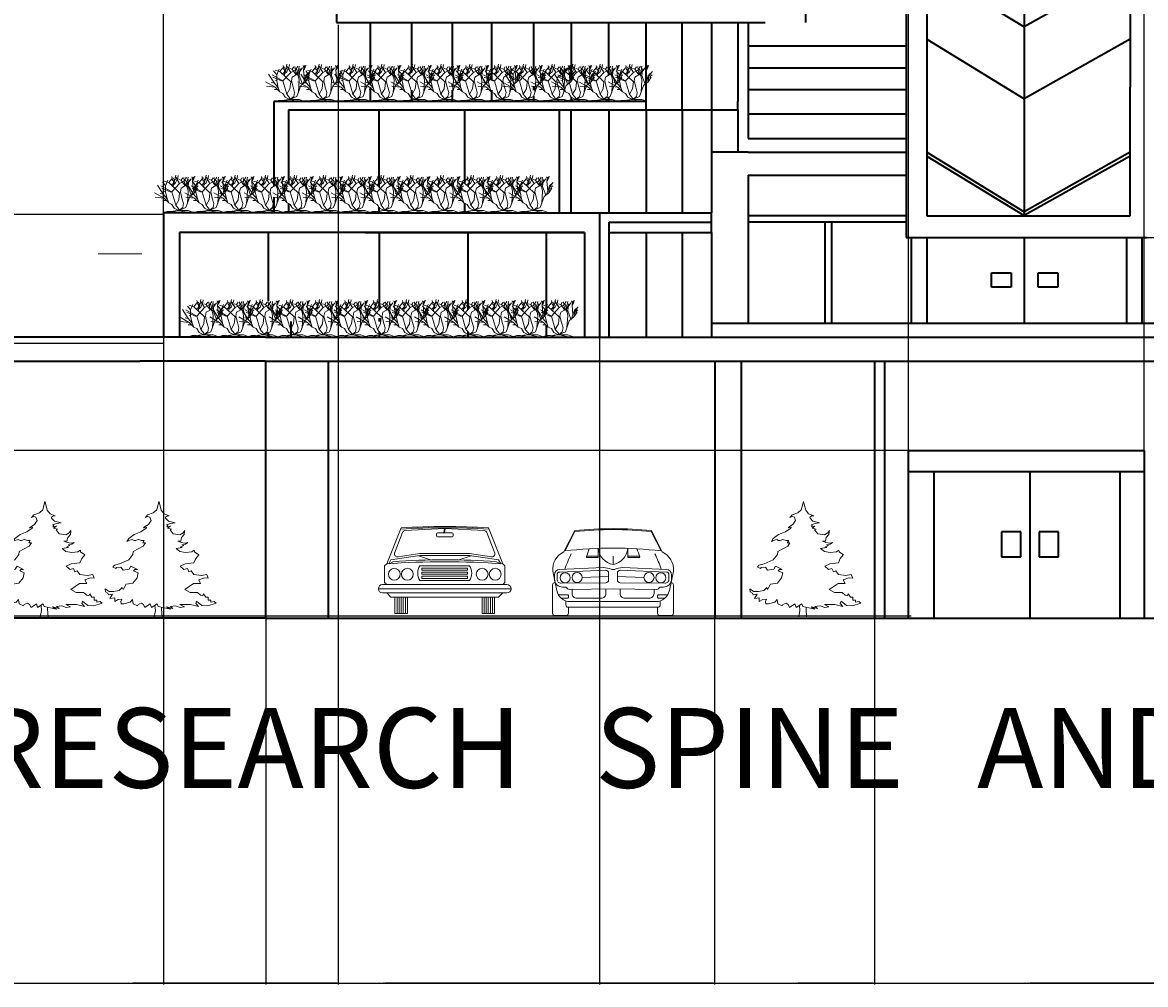
# Model space of a CAD drawing. Units: inches. Extents: x -160 to 434, y -145 to 103.
# Tile 2 of 7: x -26 to 107, y -145 to -31. Entities that reach past the tile are written whole.
import ezdxf

# ---------------------------------------------------------------- set-up
doc = ezdxf.new("R2010")
doc.units = ezdxf.units.IN
doc.header["$MEASUREMENT"] = 0
for name, color, linetype, lineweight in [('A-ANNO-DIMS', 2, 'Continuous', 18), ('A-ANNO-SYMB', 2, 'Continuous', 13), ('A-ANNO-TEXT', 3, 'Continuous', 18), ('A-ELEV', 7, 'Continuous', 35), ('A-ENTO-VEHC', 8, 'Continuous', 13), ('L-PLNT', 3, 'Continuous', 13)]:
    doc.layers.add(name, color=color, linetype=linetype, lineweight=lineweight)
doc.styles.get("Standard").update_dxf_attribs({"font": 'arial.ttf'})
doc.dimstyles.get("Standard").update_dxf_attribs({"dimtxt": 0.18, "dimasz": 0.18, "dimexe": 0.18, "dimexo": 0.0625, "dimgap": 0.09, "dimtad": 0, "dimtih": 1, "dimtoh": 1, "dimdec": 4, "dimzin": 0, "dimdsep": 46, "dimtxsty": 'Standard', "dimcen": 0.09, "dimadec": 0, "dimazin": 0, "dimtfac": 1, "dimtdec": 4, "dimtofl": 0, "dimtmove": 0, "dimatfit": 3, "dimfxl": 1, "dimtolj": 1, "dimtzin": 0, "dimarcsym": 0})

# ---------------------------------------------------------------- blocks, each defined once
blk = doc.blocks.new('*U7')
for p, q in [((-8.263, 7.598), (-8.747, 14.105)), ((-9.75, 0), (-8.263, 7.598)), ((-0.771, 9.56), (-0.69, 11.833)), ((0, 0), (-0.771, 9.56))]:
    blk.add_line(p, q)
for points in [[(-3.9, 142.35), (-6.596, 132.037), (-10.801, 128.443), (-17.81, 126.047), (-20.614, 122.452), (-17.81, 123.65), (-15.007, 123.051), (-13.605, 118.858), (-16.876, 114.065), (-21.549, 111.07), (-22.951, 109.872), (-19.212, 110.471), (-19.68, 109.273), (-26.222, 105.079), (-34.633, 101.485), (-41.175, 96.693), (-43.511, 93.098), (-41.175, 94.296), (-36.969, 95.494), (-34.633, 94.296), (-32.764, 94.296), (-29.493, 95.494)], [(-3.759, 141.97), (-1.074, 131.643), (2.437, 127.141), (8.84, 124.493), (6.568, 124.493), (4.09, 123.169), (4.296, 121.846), (7.807, 117.874), (16.069, 116.02), (10.492, 115.226), (5.535, 113.372), (6.981, 112.843), (5.948, 110.989), (10.286, 112.048), (6.775, 109.401), (11.732, 108.077), (9.873, 107.282), (13.797, 102.516), (21.852, 101.192), (25.983, 103.84), (28.048, 106.488), (27.842, 105.164), (27.429, 101.457), (24.124, 97.75), (23.091, 93.513), (19.58, 93.513), (23.505, 91.66), (28.255, 90.866), (31.973, 91.925), (29.081, 89.806), (24.537, 88.747), (26.809, 88.218), (22.472, 86.099), (24.95, 85.57), (17.308, 84.246), (21.852, 80.804), (29.081, 79.215), (36.723, 80.009), (39.821, 82.392), (40.028, 80.009), (45.398, 76.567)], [(-29.25, 95.55), (-25.287, 94.296), (-22.016, 94.296), (-23.885, 91.301), (-20.614, 91.301), (-23.418, 87.108), (-35.567, 80.518), (-36.035, 76.924), (-41.175, 70.334), (-52.389, 65.542), (-58.931, 63.744), (-60.8, 61.348), (-57.062, 59.551), (-56.128, 60.749), (-50.987, 61.348), (-48.184, 57.754), (-40.707, 58.952), (-38.371, 62.546), (-30.427, 58.353), (-33.698, 58.353), (-35.1, 56.556), (-29.493, 54.159), (-30.894, 48.169), (-36.035, 41.579), (-44.446, 40.381), (-48.184, 33.791), (-49.118, 36.188), (-52.857, 32.593), (-59.399, 31.395), (-65.473, 31.395), (-70.146, 34.39), (-69.679, 30.796), (-66.875, 28.999), (-65.941, 27.202), (-61.268, 27.801), (-64.539, 22.409), (-58.464, 23.607), (-58.464, 18.815), (-54.258, 21.211), (-49.586, 21.81), (-50.987, 18.815), (-50.52, 15.82), (-47.249, 15.82), (-39.306, 18.216), (-36.502, 21.211), (-35.567, 15.82), (-30.427, 13.423), (-29.493, 15.221), (-25.287, 17.018), (-22.951, 15.221), (-21.081, 11.626), (-14.539, 15.82), (-13.138, 11.626), (-6.128, 15.82), (-4.726, 12.824), (10.226, 9.23), (5.554, 12.225), (13.497, 10.428), (10.226, 12.824), (16.768, 13.423), (22.376, 11.626), (27.516, 12.225), (21.909, 15.221), (34.993, 15.221), (44.806, 12.824), (41.535, 16.419), (42.469, 19.414), (49.011, 14.023), (56.487, 13.423), (66.768, 17.018), (64.431, 18.815), (60.226, 18.216), (60.226, 20.612), (56.955, 20.612), (56.955, 24.206), (54.151, 24.206), (51.348, 28.4), (50.413, 26.004), (47.609, 26.603), (43.871, 30.197), (38.731, 30.197), (34.525, 30.197), (27.983, 33.791), (38.731, 40.98), (47.609, 40.98), (45.273, 45.773), (52.282, 48.169), (56.955, 47.57), (55.086, 52.362), (48.544, 51.164), (39.198, 52.362), (35.927, 56.556), (33.123, 55.357), (31.254, 59.551), (27.049, 58.353), (22.376, 62.546), (28.451, 65.542), (39.198, 66.74), (41.535, 72.131), (45.273, 76.325)]]:
    blk.add_lwpolyline(points)
blk = doc.blocks.new('*U8')
for p, q in [((-37.38, 32.04), (-28.11, 55.23)), ((-0.21, 54.74), (-0.67, 52.07)), ((0.21, 54.74), (-0.23, 52.08)), ((37.38, 32.04), (28.11, 55.23)), ((-34.71, 34.71), (-16.02, 37.38)), ((-16.94, 37.24), (-9.08, 34.62)), ((-16.02, 37.38), (0, 37.38)), ((16.02, 37.38), (0, 37.38)), ((16.93, 37.24), (9.08, 34.62)), ((34.71, 34.71), (16.02, 37.38)), ((-38.72, 30.71), (-37.38, 32.04)), ((-38.72, 20.03), (-38.72, 30.71)), ((-36.05, 32.04), (-34.71, 34.71)), ((-35.8, 32.16), (-33.38, 33.38)), ((-16.02, 30.71), (16.02, 30.71)), ((-14.69, 29.37), (14.69, 29.37)), ((-14.69, 28.04), (-14.69, 29.37)), ((14.69, 29.37), (14.69, 28.04)), ((35.8, 32.16), (33.38, 33.38)), ((34.71, 34.71), (36.05, 32.04)), ((38.72, 30.71), (37.38, 32.04)), ((38.72, 20.03), (38.72, 30.71)), ((14.69, 28.04), (-14.69, 28.04)), ((-14.69, 26.7), (14.69, 26.7)), ((-14.69, 25.37), (-14.69, 26.7)), ((14.69, 25.37), (-14.69, 25.37)), ((-14.69, 24.03), (14.69, 24.03)), ((-14.69, 22.7), (-14.69, 24.03)), ((14.69, 22.7), (-14.69, 22.7)), ((14.69, 26.7), (14.69, 25.37)), ((14.69, 24.03), (14.69, 22.7)), ((-42.72, 16.02), (42.72, 16.02)), ((-40.05, 18.69), (40.05, 18.69)), ((-37.38, 18.69), (-38.72, 20.03)), ((16.02, 21.36), (-16.02, 21.36)), ((37.38, 18.69), (38.72, 20.03)), ((40.05, 13.35), (-40.05, 13.35)), ((-37.38, 13.35), (-34.71, 10.68)), ((-34.71, 10.68), (34.71, 10.68)), ((-32.04, 10.68), (-32.04, 0)), ((-30.71, 10.68), (-30.71, 0)), ((-29.37, 0), (-29.37, 10.68)), ((-28.04, 10.68), (-28.04, 0)), ((-26.7, 0), (-26.7, 10.68)), ((-25.37, 10.68), (-25.37, 0)), ((-24.03, 0), (-24.03, 10.68)), ((24.03, 0), (24.03, 10.68)), ((25.37, 0), (25.37, 10.68)), ((26.7, 10.68), (26.7, 0)), ((28.04, 0), (28.04, 10.68)), ((29.37, 10.68), (29.37, 0)), ((30.71, 0), (30.71, 10.68)), ((32.04, 10.68), (32.04, 0)), ((34.71, 10.68), (37.38, 13.35)), ((-32.04, 0), (-24.03, 0)), ((32.04, 0), (24.03, 0))]:
    blk.add_line(p, q)
for points in [[(-27.12, 52.31), (-32.28, 38.89)], [(0, 54.74), (-25.63, 53.46)], [(-5.34, 50.07), (-5.34, 51.4)], [(-4.67, 52.07), (0, 52.07)], [(4.67, 52.07), (0, 52.07)], [(0.01, 54.74), (25.64, 53.45)], [(5.34, 50.07), (5.34, 51.4)], [(27.13, 52.3), (32.28, 38.88)], [(0, 49.4), (-4.67, 49.4)], [(0, 49.4), (4.67, 49.4)], [(-30.06, 36.56), (-16.02, 38.72), (0, 38.72)], [(30.06, 36.54), (16.02, 38.71), (0, 38.72)]]:
    blk.add_lwpolyline(points)
for centre in [(-32.47, 25.37), (-24.06, 25.37), (24.06, 25.37), (32.47, 25.37)]:
    blk.add_circle(centre, 3.8)
for centre, radius, start, end in [((0, -432), 487.32, 86.65721, 93.3419), ((0, -431.24), 487.32, 86.69396, 93.3033), ((-25.37, 51.59), 1.89, 97.4497, 154.9311), ((-4.67, 51.4), 0.668, 93.60832, 178.1081), ((4.67, 51.4), 0.668, 1.89193, 86.39168), ((25.37, 51.57), 1.89, 25.04208, 82.52346), ((-4.67, 50.07), 0.668, 184.4192, 266.4386), ((4.67, 50.07), 0.668, 273.5614, 355.5808), ((-30.43, 38.42), 1.89, 166.5724, 279.9572), ((30.43, 38.41), 1.89, 260.016, 13.40079), ((0, -490.66), 524.03, 85.90918, 94.09081), ((0.67, -399.87), 434.58, 90.08801, 94.49321), ((-8.68, 26.03), 8.7, 147.5288, 212.4712), ((-0.67, -399.87), 434.58, 85.50679, 89.91199), ((8.68, 26.03), 8.7, 327.5288, 32.47119), ((-40.05, 16.02), 2.67, 90, 270), ((40.05, 16.02), 2.67, 270, 90)]:
    blk.add_arc(centre, radius, start, end)
blk = doc.blocks.new('*U9')
for p, q in [((-9.51, 37.84), (-9.51, 43.25)), ((0, 32.82), (0, 38.19)), ((9.51, 37.84), (9.51, 43.25)), ((-19.91, 24.53), (-2.81, 25.14)), ((2.81, 25.14), (19.91, 24.53))]:
    blk.add_line(p, q)
for points in [[(-38.83, 28.63), (-36.22, 16.07, 0.355359), (-27.52, 9), (27.58, 9, 0.355331), (36.28, 16.07), (38.89, 28.63, 0.324597), (31.68, 40.93), (24.69, 54.68, 0.052145), (-24.63, 54.68), (-31.63, 40.93, 0.324597)], [(-24.58, 54.09), (-30.92, 41.61), (-30.92, 41.61, -0.059427), (30.98, 41.61), (24.64, 54.09, 0.05217)], [(-16.8, 37.38), (-9.88, 37.38, 0.414214), (-9.51, 37.75), (-9.51, 37.82, 0.414214), (-9.88, 38.19), (-16.8, 38.19, 0.414214), (-17.17, 37.82), (-17.17, 37.75, 0.414214)], [(16.8, 37.38), (9.88, 37.38, -0.414214), (9.51, 37.75), (9.51, 37.82, -0.414214), (9.88, 38.19), (16.8, 38.19, -0.414214), (17.17, 37.82), (17.17, 37.75, -0.414214)], [(-4.66, 29.17, -0.427329), (-2.81, 27.41), (-2.81, 22.88, -0.410558), (-4.56, 21.11), (-33.36, 20.8, -0.417878), (-36.04, 23.45), (-36.04, 26.26, -0.401219), (-34.35, 28.03)], [(4.66, 29.17, 0.427329), (2.81, 27.41), (2.81, 22.88, 0.410558), (4.56, 21.11), (33.36, 20.8, 0.417878), (36.04, 23.45), (36.04, 26.26, 0.401219), (34.35, 28.03)]]:
    blk.add_lwpolyline(points, format="xyb", close=True)
for points in [[(-6.29, 30.92), (-34.43, 29.71, 0.401219), (-37.73, 26.26), (-37.73, 23.63, 0.414214), (-32.43, 18.34), (-31.07, 18.34, -0.198912), (-29.82, 17.82), (-29.29, 17.29, 0.202778), (-28.01, 16.77), (0, 17.13), (28.01, 16.77, 0.202778), (29.29, 17.29), (29.82, 17.82, -0.198912), (31.07, 18.34), (32.43, 18.34, 0.414214), (37.73, 23.63), (37.73, 26.26, 0.401219), (34.43, 29.71), (6.29, 30.92)], [(6.29, 30.92, 0.105807), (0.87, 29.72, -0.131652), (-0.87, 29.72, 0.105807), (-6.29, 30.92)], [(-28.7, 5.37), (-28.7, 1.48, -0.414214), (-30.18, 0), (-37.41, 0, -0.414214), (-38.89, 1.48), (-38.89, 19.74, -0.414214), (-37.41, 21.22), (-37.29, 21.22)], [(-4.56, 17.07), (-4.56, 14.1, -0.414214), (-7.52, 11.14), (-23.43, 11.14, -0.414214), (-26.39, 14.1), (-26.39, 16.79)], [(4.56, 17.07), (4.56, 14.1, 0.414214), (7.52, 11.14), (23.43, 11.14, 0.414214), (26.39, 14.1), (26.39, 16.79)], [(28.7, 5.37), (28.7, 1.48, 0.414214), (30.18, 0), (37.41, 0, 0.414214), (38.89, 1.48), (38.89, 19.74, 0.414214), (37.41, 21.22), (37.35, 21.22)], [(-35.17, 13.37), (-29.44, 13.37, -0.414214), (-28.7, 12.63), (-28.7, 11.88, -0.414214), (-29.44, 11.14), (-33.31, 11.14)], [(-30.39, 9.47), (-30.39, 6.85, 0.414214), (-28.91, 5.37), (28.91, 5.37, 0.414214), (30.39, 6.85), (30.39, 9.47)], [(35.17, 13.37), (29.44, 13.37, 0.414214), (28.7, 12.63), (28.7, 11.88, 0.414214), (29.44, 11.14), (33.31, 11.14)]]:
    blk.add_lwpolyline(points, format="xyb")
for centre in [(-30.79, 24.36), (-23.15, 24.53), (23.15, 24.53), (30.79, 24.36)]:
    blk.add_circle(centre, 3.24)
for centre, radius, start, end in [((27.74, 11.77), 61.38, 152.82966, 162.90143), ((41.5, 19.77), 61.38, 157.83365, 162.90143), ((2.03, 44.22), 11.58, 184.78179, 259.90449), ((-2.03, 44.22), 11.58, 280.09551, 355.21821), ((-41.5, 19.77), 61.38, 17.09857, 22.16635), ((-27.69, 11.77), 61.38, 17.09857, 27.17034)]:
    blk.add_arc(centre, radius, start, end)
blk = doc.blocks.new('*U5')
for p, q in [((-12.471, 19.775), (-12.898, 22.044)), ((-11.28, 19.619), (-12.104, 21.184)), ((-11.433, 18.289), (-10.457, 22.749)), ((-8.16, 17.76), (-10.56, 21.6)), ((-9.48, 19.775), (-8.992, 22.592)), ((-7.2, 19.68), (-6.24, 21.12)), ((-5.086, 17.741), (-5.513, 21.34)), ((-5.28, 19.2), (-3.84, 21.6)), ((-3.377, 18.602), (-2.888, 21.575)), ((-0.508, 21.888), (-0.081, 20.558)), ((-0.203, 19.149), (0.102, 21.34)), ((-0.02, 20.01), (0.896, 21.105)), ((0.041, 20.714), (1.384, 22.044)), ((0.102, 21.34), (0.835, 21.888)), ((-18.24, 11.04), (-21.755, 16.655)), ((-12.96, 12.48), (-19.68, 16.32)), ((-13.92, 12.48), (-19.2, 14.88)), ((-16.8, 16.32), (-18.72, 18.72)), ((-14.88, 18.24), (-17.76, 19.2)), ((-16.8, 16.32), (-15.36, 19.68)), ((-16.8, 12.48), (-16.8, 16.32)), ((-14.88, 18.24), (-12.96, 20.64)), ((-8.16, 12), (-14.88, 18.24)), ((-13.325, 16.724), (-11.433, 18.289)), ((-12.96, 12.48), (-8.16, 17.76)), ((-11.677, 19.071), (-12.471, 19.775)), ((-12.043, 15.628), (-11.921, 18.836)), ((-11.982, 16.802), (-10.579, 18.054)), ((-11.921, 18.836), (-10.64, 20.401)), ((-10.579, 18.054), (-9.846, 19.697)), ((-7.2, 19.68), (-8.64, 20.16)), ((-8.16, 17.76), (-5.28, 19.2)), ((-7.68, 12.48), (-7.2, 14.88)), ((-4.8, 16.32), (-7.2, 19.68)), ((-7.2, 14.88), (-3.84, 16.8)), ((-3.377, 15.315), (-5.086, 17.819)), ((-2.88, 12.96), (-4.32, 19.68)), ((-3.84, 16.8), (-0.96, 20.64)), ((-2.766, 16.802), (-3.377, 18.602)), ((-2.88, 15.84), (-2.4, 20.16)), ((-0.96, 10.56), (-2.88, 15.84)), ((0.346, 13.203), (-0.203, 19.149)), ((-0.142, 19.384), (0.59, 20.401)), ((0.346, 13.203), (1.323, 16.254)), ((0.96, 12), (1.44, 15.36)), ((0.96, 12), (2.88, 14.88)), ((1.323, 16.254), (3.642, 18.289)), ((1.44, 15.36), (2.88, 17.28)), ((1.92, 13.44), (2.4, 15.36)), ((2.4, 15.36), (3.36, 16.32)), ((-17.76, 8.64), (-23.663, 11.961)), ((-17.76, 8.64), (-23.128, 9.222)), ((-18.24, 11.04), (-20.16, 11.52)), ((-15.84, 8.16), (-18.24, 11.04)), ((-16.32, 7.2), (-18.24, 7.2)), ((-16.8, 12.48), (-17.76, 12.96)), ((-14.88, 5.76), (-17.76, 8.64)), ((-15.84, 8.16), (-16.8, 12.48)), ((-14.88, 5.76), (-15.84, 8.16)), ((-12.96, 12.48), (-13.92, 12.48)), ((-10.56, 4.32), (-12.96, 12.48)), ((-10.56, 4.32), (-8.64, 7.68)), ((-8.64, 7.68), (-8.16, 12)), ((-6.72, 8.64), (-7.68, 12.48)), ((-5.76, 5.28), (-6.72, 8.64)), ((-4.32, 2.88), (-1.92, 9.6)), ((-3.36, 5.28), (-2.88, 12.96)), ((-1.92, 9.6), (0.96, 12)), ((-0.48, 10.8), (0.346, 13.203)), ((-15.84, 0.48), (-17.76, 0)), ((-13.44, 0.48), (-15.84, 0.48)), ((-12.96, 4.8), (-14.88, 5.76)), ((-9.6, 0.96), (-13.44, 0.48)), ((-11.52, 2.4), (-12.96, 4.8)), ((-9.6, 0.96), (-12.96, 0)), ((-8.64, 0.96), (-11.52, 2.4)), ((-8.64, 1.92), (-10.56, 4.32)), ((-9.6, 0.96), (-7.68, 0.96)), ((-8.64, 0.96), (-4.32, 2.88)), ((-8.64, 0.96), (-6.24, 2.88)), ((-8.64, 0.96), (-8.64, 1.92)), ((-8.64, 0.96), (-2.88, 0.96)), ((-7.68, 0.96), (-6.24, 0.48)), ((-6.24, 2.88), (-5.76, 5.28)), ((-6.24, 0.48), (-3.36, 0)), ((-2.88, 0.96), (0, 0))]:
    blk.add_line(p, q)
blk = doc.blocks.new('*D12')
at = {"layer": 'A-ANNO-DIMS', "color": 0, "lineweight": -2, "transparency": 16777216}
for p, q in [((-84.07, -101.41), (-84.07, -144.81)), ((403.75, -101.41), (403.75, -144.81)), ((-83.89, -144.63), (159.44, -144.63)), ((403.57, -144.63), (160.24, -144.63))]:
    blk.add_line(p, q, dxfattribs=at)
at = {"layer": 'A-ANNO-DIMS', "color": 0, "transparency": 16777216}
for points in [[(-83.89, -144.6), (-83.89, -144.66), (-84.07, -144.63)], [(403.57, -144.6), (403.57, -144.66), (403.75, -144.63)]]:
    blk.add_solid(points, dxfattribs=at)
at = {"layer": 'Defpoints', "color": 0, "transparency": 16777216}
for p in [(-84.07, -101.35), (403.75, -101.35), (403.75, -144.63)]:
    blk.add_point(p, dxfattribs=at)
at = {"layer": 'A-ANNO-DIMS', "color": 0, "transparency": 16777216, "insert": (159.84, -144.63), "char_height": 0.18, "attachment_point": 5}
blk.add_mtext('\\A1;487.8', dxfattribs=at)
blk = doc.blocks.new('*D15')
at = {"layer": 'A-ANNO-DIMS', "color": 0, "lineweight": -2, "transparency": 16777216}
for p, q in [((2.83, 44.89), (-114.3, 44.89)), ((-114.12, 44.71), (-114.12, -28.36)), ((-114.12, -101.79), (-114.12, -28.72)), ((-29.6, -101.97), (-114.3, -101.97))]:
    blk.add_line(p, q, dxfattribs=at)
at = {"layer": 'A-ANNO-DIMS', "color": 0, "transparency": 16777216}
for points in [[(-114.15, 44.71), (-114.09, 44.71), (-114.12, 44.89)], [(-114.15, -101.79), (-114.09, -101.79), (-114.12, -101.97)]]:
    blk.add_solid(points, dxfattribs=at)
at = {"layer": 'Defpoints', "color": 0, "transparency": 16777216}
for p in [(-114.12, 44.89), (2.89, 44.89), (-29.54, -101.97)]:
    blk.add_point(p, dxfattribs=at)
at = {"layer": 'A-ANNO-DIMS', "color": 0, "transparency": 16777216, "insert": (-114.12, -28.54), "char_height": 0.18, "attachment_point": 5}
blk.add_mtext('\\A1;146.87', dxfattribs=at)
blk = doc.blocks.new('*D16')
at = {"layer": 'A-ANNO-DIMS', "color": 0, "lineweight": -2, "transparency": 16777216}
for p, q in [((-29.54, -102.04), (-29.54, -144.81)), ((2.66, -101.41), (2.66, -144.81)), ((-29.36, -144.63), (-13.76, -144.63)), ((2.48, -144.63), (-13.12, -144.63))]:
    blk.add_line(p, q, dxfattribs=at)
at = {"layer": 'A-ANNO-DIMS', "color": 0, "transparency": 16777216}
for points in [[(-29.36, -144.6), (-29.36, -144.66), (-29.54, -144.63)], [(2.48, -144.6), (2.48, -144.66), (2.66, -144.63)]]:
    blk.add_solid(points, dxfattribs=at)
at = {"layer": 'Defpoints', "color": 0, "transparency": 16777216}
for p in [(-29.54, -101.97), (2.66, -101.35), (2.66, -144.63)]:
    blk.add_point(p, dxfattribs=at)
at = {"layer": 'A-ANNO-DIMS', "color": 0, "transparency": 16777216, "insert": (-13.44, -144.63), "char_height": 0.18, "attachment_point": 5}
blk.add_mtext('\\A1;32.2', dxfattribs=at)
blk = doc.blocks.new('*D17')
at = {"layer": 'A-ANNO-DIMS', "color": 0, "lineweight": -2, "transparency": 16777216}
for p, q in [((2.66, -101.41), (2.66, -144.81)), ((55.95, -101.41), (55.95, -144.81)), ((2.84, -144.63), (28.91, -144.63)), ((55.77, -144.63), (29.7, -144.63))]:
    blk.add_line(p, q, dxfattribs=at)
at = {"layer": 'A-ANNO-DIMS', "color": 0, "transparency": 16777216}
for points in [[(2.84, -144.6), (2.84, -144.66), (2.66, -144.63)], [(55.77, -144.6), (55.77, -144.66), (55.95, -144.63)]]:
    blk.add_solid(points, dxfattribs=at)
at = {"layer": 'Defpoints', "color": 0, "transparency": 16777216}
for p in [(2.66, -101.35), (55.95, -101.35), (55.95, -144.63)]:
    blk.add_point(p, dxfattribs=at)
at = {"layer": 'A-ANNO-DIMS', "color": 0, "transparency": 16777216, "insert": (29.3, -144.63), "char_height": 0.18, "attachment_point": 5}
blk.add_mtext('\\A1;53.29', dxfattribs=at)
blk = doc.blocks.new('*D18')
at = {"layer": 'A-ANNO-DIMS', "color": 0, "lineweight": -2, "transparency": 16777216}
for p, q in [((55.95, -101.41), (55.95, -144.81)), ((74.92, -101.41), (74.92, -144.81)), ((56.13, -144.63), (65.05, -144.63)), ((74.74, -144.63), (65.82, -144.63))]:
    blk.add_line(p, q, dxfattribs=at)
at = {"layer": 'A-ANNO-DIMS', "color": 0, "transparency": 16777216}
for points in [[(56.13, -144.6), (56.13, -144.66), (55.95, -144.63)], [(74.74, -144.6), (74.74, -144.66), (74.92, -144.63)]]:
    blk.add_solid(points, dxfattribs=at)
at = {"layer": 'Defpoints', "color": 0, "transparency": 16777216}
for p in [(55.95, -101.35), (74.92, -101.35), (74.92, -144.63)]:
    blk.add_point(p, dxfattribs=at)
at = {"layer": 'A-ANNO-DIMS', "color": 0, "transparency": 16777216, "insert": (65.44, -144.63), "char_height": 0.18, "attachment_point": 5}
blk.add_mtext('\\A1;18.97', dxfattribs=at)
blk = doc.blocks.new('*D19')
at = {"layer": 'A-ANNO-DIMS', "color": 0, "lineweight": -2, "transparency": 16777216}
for p, q in [((74.92, -101.41), (74.92, -144.81)), ((111.05, -101.41), (111.05, -144.81)), ((75.1, -144.63), (92.59, -144.63)), ((110.87, -144.63), (93.38, -144.63))]:
    blk.add_line(p, q, dxfattribs=at)
at = {"layer": 'A-ANNO-DIMS', "color": 0, "transparency": 16777216}
for points in [[(75.1, -144.6), (75.1, -144.66), (74.92, -144.63)], [(110.87, -144.6), (110.87, -144.66), (111.05, -144.63)]]:
    blk.add_solid(points, dxfattribs=at)
at = {"layer": 'Defpoints', "color": 0, "transparency": 16777216}
for p in [(74.92, -101.35), (111.05, -101.35), (111.05, -144.63)]:
    blk.add_point(p, dxfattribs=at)
at = {"layer": 'A-ANNO-DIMS', "color": 0, "transparency": 16777216, "insert": (92.98, -144.63), "char_height": 0.18, "attachment_point": 5}
blk.add_mtext('\\A1;36.12', dxfattribs=at)
blk = doc.blocks.new('*D24')
at = {"layer": 'A-ANNO-DIMS', "color": 0, "lineweight": -2, "transparency": 16777216}
for p, q in [((78.96, -81.39), (78.96, 102.5)), ((79.14, 102.32), (92.54, 102.32)), ((106.73, 102.32), (93.33, 102.32)), ((106.91, -81.39), (106.91, 102.5))]:
    blk.add_line(p, q, dxfattribs=at)
at = {"layer": 'A-ANNO-DIMS', "color": 0, "transparency": 16777216}
for points in [[(79.14, 102.35), (79.14, 102.29), (78.96, 102.32)], [(106.73, 102.35), (106.73, 102.29), (106.91, 102.32)]]:
    blk.add_solid(points, dxfattribs=at)
at = {"layer": 'Defpoints', "color": 0, "transparency": 16777216}
for p in [(106.91, 102.32), (78.96, -81.45), (106.91, -81.45)]:
    blk.add_point(p, dxfattribs=at)
at = {"layer": 'A-ANNO-DIMS', "color": 0, "transparency": 16777216, "insert": (92.94, 102.32), "char_height": 0.18, "attachment_point": 5}
blk.add_mtext('\\A1;27.95', dxfattribs=at)
blk = doc.blocks.new('*D25')
at = {"layer": 'A-ANNO-DIMS', "color": 0, "lineweight": -2, "transparency": 16777216}
for p, q in [((78.9, -81.45), (-114.3, -81.45)), ((-114.12, -81.63), (-114.12, -91.1)), ((-114.12, -100.92), (-114.12, -91.46)), ((79.28, -101.1), (-114.3, -101.1))]:
    blk.add_line(p, q, dxfattribs=at)
at = {"layer": 'A-ANNO-DIMS', "color": 0, "transparency": 16777216}
for points in [[(-114.15, -81.63), (-114.09, -81.63), (-114.12, -81.45)], [(-114.15, -100.92), (-114.09, -100.92), (-114.12, -101.1)]]:
    blk.add_solid(points, dxfattribs=at)
at = {"layer": 'Defpoints', "color": 0, "transparency": 16777216}
for p in [(78.96, -81.45), (-114.12, -101.1), (79.34, -101.1)]:
    blk.add_point(p, dxfattribs=at)
at = {"layer": 'A-ANNO-DIMS', "color": 0, "transparency": 16777216, "insert": (-114.12, -91.28), "char_height": 0.18, "attachment_point": 5}
blk.add_mtext('\\A1;19.646', dxfattribs=at)
blk = doc.blocks.new('*D30')
at = {"layer": 'A-ANNO-DIMS', "color": 0, "lineweight": -2, "transparency": 16777216}
for p, q in [((2.83, 3.66), (-114.3, 3.66)), ((-114.12, 3.48), (-114.12, -32.35)), ((-114.12, -68.55), (-114.12, -32.72)), ((-9.37, -68.73), (-114.3, -68.73))]:
    blk.add_line(p, q, dxfattribs=at)
at = {"layer": 'A-ANNO-DIMS', "color": 0, "transparency": 16777216}
for points in [[(-114.15, 3.48), (-114.09, 3.48), (-114.12, 3.66)], [(-114.15, -68.55), (-114.09, -68.55), (-114.12, -68.73)]]:
    blk.add_solid(points, dxfattribs=at)
at = {"layer": 'Defpoints', "color": 0, "transparency": 16777216}
for p in [(-114.12, 3.66), (2.89, 3.66), (-9.31, -68.73)]:
    blk.add_point(p, dxfattribs=at)
at = {"layer": 'A-ANNO-DIMS', "color": 0, "transparency": 16777216, "insert": (-114.12, -32.54), "char_height": 0.18, "attachment_point": 5}
blk.add_mtext('\\A1;72.4', dxfattribs=at)
blk = doc.blocks.new('*D32')
at = {"layer": 'A-ANNO-DIMS', "color": 0, "lineweight": -2, "transparency": 16777216}
for p, q in [((107.33, -56.17), (433.98, -56.17)), ((433.8, -56.35), (433.8, -61.07)), ((433.8, -66.15), (433.8, -61.43)), ((106.73, -66.33), (433.98, -66.33))]:
    blk.add_line(p, q, dxfattribs=at)
at = {"layer": 'A-ANNO-DIMS', "color": 0, "transparency": 16777216}
for points in [[(433.77, -56.35), (433.83, -56.35), (433.8, -56.17)], [(433.77, -66.15), (433.83, -66.15), (433.8, -66.33)]]:
    blk.add_solid(points, dxfattribs=at)
at = {"layer": 'Defpoints', "color": 0, "transparency": 16777216}
for p in [(107.27, -56.17), (106.67, -66.33), (433.8, -66.33)]:
    blk.add_point(p, dxfattribs=at)
at = {"layer": 'A-ANNO-DIMS', "color": 0, "transparency": 16777216, "insert": (433.8, -61.25), "char_height": 0.18, "attachment_point": 5}
blk.add_mtext('\\A1;10.165', dxfattribs=at)
blk = doc.blocks.new('*D35')
at = {"layer": 'A-ANNO-DIMS', "color": 0, "lineweight": -2, "transparency": 16777216}
for p, q in [((42.27, -53.31), (42.27, -144.81)), ((-9.45, -53.49), (-9.45, -144.81)), ((-9.27, -144.63), (16.02, -144.63)), ((42.09, -144.63), (16.8, -144.63))]:
    blk.add_line(p, q, dxfattribs=at)
at = {"layer": 'A-ANNO-DIMS', "color": 0, "transparency": 16777216}
for points in [[(-9.27, -144.6), (-9.27, -144.66), (-9.45, -144.63)], [(42.09, -144.6), (42.09, -144.66), (42.27, -144.63)]]:
    blk.add_solid(points, dxfattribs=at)
at = {"layer": 'Defpoints', "color": 0, "transparency": 16777216}
for p in [(42.27, -53.24), (-9.45, -53.43), (42.27, -144.63)]:
    blk.add_point(p, dxfattribs=at)
at = {"layer": 'A-ANNO-DIMS', "color": 0, "transparency": 16777216, "insert": (16.41, -144.63), "char_height": 0.18, "attachment_point": 5}
blk.add_mtext('\\A1;51.72', dxfattribs=at)
blk = doc.blocks.new('*D36')
at = {"layer": 'A-ANNO-DIMS', "color": 0, "lineweight": -2, "transparency": 16777216}
for p, q in [((-9.51, -53.43), (-114.3, -53.43)), ((-114.12, -53.61), (-114.12, -60.9)), ((-114.12, -68.55), (-114.12, -61.26)), ((-9.37, -68.73), (-114.3, -68.73))]:
    blk.add_line(p, q, dxfattribs=at)
at = {"layer": 'A-ANNO-DIMS', "color": 0, "transparency": 16777216}
for points in [[(-114.15, -53.61), (-114.09, -53.61), (-114.12, -53.43)], [(-114.15, -68.55), (-114.09, -68.55), (-114.12, -68.73)]]:
    blk.add_solid(points, dxfattribs=at)
at = {"layer": 'Defpoints', "color": 0, "transparency": 16777216}
for p in [(-9.45, -53.43), (-114.12, -68.73), (-9.31, -68.73)]:
    blk.add_point(p, dxfattribs=at)
at = {"layer": 'A-ANNO-DIMS', "color": 0, "transparency": 16777216, "insert": (-114.12, -61.08), "char_height": 0.18, "attachment_point": 5}
blk.add_mtext('\\A1;15.304', dxfattribs=at)
blk = doc.blocks.new('*D37')
at = {"layer": 'A-ANNO-DIMS', "color": 0, "lineweight": -2, "transparency": 16777216}
for p, q in [((11.28, -30.92), (11.28, -144.81)), ((-9.45, -53.49), (-9.45, -144.81)), ((-9.27, -144.63), (0.52, -144.63)), ((11.1, -144.63), (1.31, -144.63))]:
    blk.add_line(p, q, dxfattribs=at)
at = {"layer": 'A-ANNO-DIMS', "color": 0, "transparency": 16777216}
for points in [[(-9.27, -144.6), (-9.27, -144.66), (-9.45, -144.63)], [(11.1, -144.6), (11.1, -144.66), (11.28, -144.63)]]:
    blk.add_solid(points, dxfattribs=at)
at = {"layer": 'Defpoints', "color": 0, "transparency": 16777216}
for p in [(11.28, -30.86), (-9.45, -53.43), (11.28, -144.63)]:
    blk.add_point(p, dxfattribs=at)
at = {"layer": 'A-ANNO-DIMS', "color": 0, "transparency": 16777216, "insert": (0.92, -144.63), "char_height": 0.18, "attachment_point": 5}
blk.add_mtext('\\A1;20.73', dxfattribs=at)
blk = doc.blocks.new('*D47')
at = {"layer": 'A-ANNO-DIMS', "color": 0, "lineweight": -2, "transparency": 16777216}
for p, q in [((-30.07, -67.91), (-30.07, 102.5)), ((-29.89, 102.32), (-20.23, 102.32)), ((-9.63, 102.32), (-19.3, 102.32)), ((-9.45, -53.37), (-9.45, 102.5))]:
    blk.add_line(p, q, dxfattribs=at)
at = {"layer": 'A-ANNO-DIMS', "color": 0, "transparency": 16777216}
for points in [[(-29.89, 102.35), (-29.89, 102.29), (-30.07, 102.32)], [(-9.63, 102.35), (-9.63, 102.29), (-9.45, 102.32)]]:
    blk.add_solid(points, dxfattribs=at)
at = {"layer": 'Defpoints', "color": 0, "transparency": 16777216}
for p in [(-9.45, 102.32), (-9.45, -53.43), (-30.07, -67.97)]:
    blk.add_point(p, dxfattribs=at)
at = {"layer": 'A-ANNO-DIMS', "color": 0, "transparency": 16777216, "insert": (-19.76, 102.32), "char_height": 0.18, "attachment_point": 5}
blk.add_mtext('\\A1;20.625', dxfattribs=at)

msp = doc.modelspace()

# ---------------------------------------------------------------- linework, layer by layer
at = {"layer": 'A-ANNO-SYMB'}
msp.add_line((-17.2202, -58.1074), (-12.0372, -58.1074), dxfattribs=at)
at = {"layer": 'A-ELEV'}
for p, q in [((105.2782, 6.4991), (105.2782, -38.311)), ((78.691, -2.0014), (78.691, -56.1669)), ((81.1405, -2.0014), (81.1405, -53.5674)), ((92.6738, -2.0014), (92.6738, -53.5674)), ((11.0861, -9.1182), (11.0861, -30.6379)), ((66.7815, -30.6379), (66.7815, -24.7325)), ((81.1405, -24.1029), (92.6738, -31.1677)), ((105.2782, -24.1029), (92.6738, -31.1677)), ((11.0861, -30.6379), (61.9316, -30.6379)), ((15.067, -30.6379), (15.067, -37.2498)), ((19.9544, -30.6379), (19.9544, -36.5858)), ((24.8102, -30.6379), (24.8102, -36.9732)), ((29.4459, -30.6379), (29.4459, -37.4933)), ((34.4496, -30.6379), (34.4496, -36.7871)), ((38.9382, -30.6379), (38.9382, -37.5554)), ((43.3532, -30.6379), (43.3532, -36.908)), ((47.7681, -30.6379), (47.7681, -38.6671)), ((47.7681, -30.6379), (47.7681, -41.0229)), ((52.036, -30.6379), (52.036, -38.6671)), ((52.036, -30.6379), (52.036, -41.0229)), ((55.5639, -30.6379), (55.5639, -53.2447)), ((58.6862, -30.6379), (58.6862, -38.6671)), ((59.9278, -30.6379), (59.9278, -38.6671)), ((81.1405, -32.6275), (92.6738, -39.6923)), ((105.2782, -32.6275), (92.6738, -39.6923)), ((59.9278, -33.4031), (78.691, -33.4031)), ((19.9544, -37.1469), (19.9544, -37.1737)), ((59.9278, -36.0223), (78.691, -36.0223)), ((15.067, -37.4944), (15.067, -37.9924)), ((15.067, -38.3382), (15.067, -38.6671)), ((24.8102, -37.9411), (24.8102, -38.2411)), ((34.4496, -38.2245), (34.4496, -38.6671)), ((38.9382, -38.6392), (38.9382, -38.6671)), ((59.9278, -38.6), (78.691, -38.6)), ((105.2782, -53.5674), (105.2782, -38.311)), ((15.067, -38.6671), (15.067, -40.0106)), ((19.9544, -38.6671), (19.9544, -40.0106)), ((24.8102, -38.6671), (24.8102, -40.0106)), ((29.4459, -38.6671), (29.4459, -40.0106)), ((34.4496, -39.3781), (34.4496, -40.0106)), ((38.9382, -39.5312), (38.9382, -40.0106)), ((43.3532, -39.508), (43.3532, -40.0106)), ((58.6862, -38.6671), (58.6862, -40.0106)), ((59.9278, -38.6671), (59.9278, -44.3998)), ((3.6399, -40.0106), (3.6399, -41.0229)), ((47.7681, -40.0106), (3.6399, -40.0106)), ((3.6399, -41.0229), (3.6399, -50.073)), ((5.3878, -41.0229), (47.7681, -41.0229)), ((5.3878, -41.0229), (5.3878, -49.8008)), ((16.0957, -41.0229), (16.0957, -50.1598)), ((26.2769, -41.0229), (26.2769, -49.7194)), ((37.5113, -41.0229), (37.5113, -53.2447)), ((38.9382, -53.2447), (38.9382, -41.0229)), ((43.4443, -53.2447), (43.4443, -41.0229)), ((47.7681, -41.0229), (58.6862, -41.0229)), ((47.8728, -53.2447), (47.8728, -41.0229)), ((52.1459, -53.2447), (52.1459, -41.0229)), ((58.6862, -41.0229), (58.6862, -40.0106)), ((58.6862, -41.0229), (58.6862, -46.0109)), ((59.9278, -41.4999), (78.691, -41.4999)), ((59.9278, -44.3998), (78.691, -44.3998)), ((59.9278, -46.0109), (55.5639, -46.0109)), ((59.9278, -46.0109), (78.691, -46.0109)), ((81.1405, -46.03), (92.6738, -53.0948)), ((81.1405, -46.4882), (92.6738, -53.553)), ((105.2782, -46.03), (92.6738, -53.0948)), ((105.2782, -46.4882), (92.6738, -53.553)), ((59.9278, -48.7744), (59.9278, -66.3322)), ((59.9278, -48.7744), (78.691, -48.7744)), ((5.3878, -50.6359), (5.3878, -50.7427)), ((26.2769, -50.5858), (26.2769, -50.7029)), ((3.6399, -51.3759), (3.6399, -53.2447)), ((14.4937, -53.2447), (-9.473, -53.2447)), ((-6.3978, -53.2447), (-9.473, -53.2447)), ((-9.473, -53.2447), (-9.473, -67.9742)), ((3.6399, -52.675), (3.6399, -53.2447)), ((5.3878, -52.1272), (5.3878, -53.2447)), ((14.4937, -53.2447), (42.2691, -53.2447)), ((16.0957, -52.5428), (16.0957, -53.2447)), ((26.2769, -52.0834), (26.2769, -53.2447)), ((42.2691, -53.2447), (42.2691, -67.9742)), ((42.2691, -53.2447), (55.5639, -53.2447)), ((55.5639, -55.5766), (55.5639, -53.2447)), ((43.4443, -54.3521), (55.5639, -54.3521)), ((43.4443, -55.5766), (43.4443, -54.3521)), ((78.691, -53.5674), (59.9278, -53.5674)), ((78.691, -54.3391), (59.9278, -54.3391)), ((69.0088, -54.3391), (69.0088, -66.3322)), ((69.8034, -54.3391), (69.8034, -66.3322)), ((81.1405, -53.5674), (105.2782, -53.5674)), ((-7.5654, -55.5766), (-7.5654, -67.9742)), ((40.5131, -55.5766), (-7.5654, -55.5766)), ((-6.3978, -55.5766), (-6.9454, -55.5766)), ((2.9669, -55.5766), (2.9669, -63.7195)), ((14.4937, -55.5766), (40.5131, -55.5766)), ((16.1323, -55.5766), (16.1323, -64.7192)), ((26.6646, -55.5766), (26.6646, -64.703)), ((35.9681, -55.5766), (35.9681, -64.4967)), ((40.5131, -55.5766), (40.5131, -67.9742)), ((43.4443, -67.9742), (43.4443, -55.5766)), ((43.4443, -55.5766), (55.5639, -55.5766)), ((47.8728, -67.9742), (47.8728, -55.5766)), ((52.1459, -67.9742), (52.1459, -55.5766)), ((55.5639, -55.5766), (55.5639, -67.9742)), ((78.691, -56.1669), (107.2684, -56.1669)), ((79.2907, -56.1669), (79.2907, -66.3322)), ((81.1405, -56.1669), (81.1405, -66.3322)), ((92.6738, -56.1669), (92.6738, -66.3322)), ((104.8174, -56.1669), (104.8174, -66.3322)), ((106.6672, -56.1669), (106.6672, -66.3322)), ((88.7955, -60.3692), (91.1349, -60.3692)), ((88.7955, -62.0486), (88.7955, -60.3692)), ((91.1349, -60.3692), (91.1349, -62.0486)), ((94.3434, -60.3692), (96.6827, -60.3692)), ((94.3434, -62.0486), (94.3434, -60.3692)), ((96.6827, -60.3692), (96.6827, -62.0486)), ((91.1349, -62.0486), (88.7955, -62.0486)), ((96.6827, -62.0486), (94.3434, -62.0486)), ((3.9379, -64.8024), (3.9379, -65.8042)), ((35.9681, -65.0634), (35.9681, -65.084)), ((-7.5654, -65.6451), (-7.5654, -67.9742)), ((5.6473, -66.1157), (5.6473, -67.9845)), ((16.1323, -65.7443), (16.1323, -66.1335)), ((35.9681, -66.5457), (35.9681, -67.9742)), ((55.5639, -66.3322), (131.6105, -66.3322)), ((-12.2824, -67.9742), (-30.0745, -67.9742)), ((2.6577, -67.9742), (-12.2824, -67.9742)), ((2.6577, -67.9742), (206.9244, -67.9742)), ((2.9669, -67.4341), (2.9669, -67.9742)), ((16.1323, -67.342), (16.1323, -67.9742)), ((26.6646, -67.3028), (26.6646, -67.9742)), ((-30.0745, -70.8373), (-12.2824, -70.8373)), ((2.6577, -70.8373), (-12.2824, -70.8373)), ((2.6577, -70.8373), (206.9244, -70.8373)), ((2.6577, -70.8373), (2.6577, -101.346)), ((10.0595, -70.8373), (10.0595, -101.346)), ((55.9512, -70.8373), (55.9512, -101.346)), ((59.0997, -70.8373), (59.0997, -101.346)), ((74.9222, -70.8373), (74.9222, -101.346)), ((76.1164, -70.8373), (76.1164, -101.346)), ((78.9633, -101.346), (78.9633, -81.4546)), ((78.9633, -81.4546), (106.9124, -81.4546)), ((106.9124, -81.4546), (106.9124, -101.346)), ((78.9633, -83.9177), (106.9124, -83.9177)), ((82.0165, -101.346), (82.0165, -83.9177)), ((93.4076, -101.346), (93.4076, -83.9177)), ((104.094, -101.346), (104.094, -83.9177)), ((89.9978, -91.0851), (89.9978, -94.0578)), ((92.3044, -91.0851), (89.9978, -91.0851)), ((92.3044, -94.0578), (92.3044, -91.0851)), ((94.4622, -91.0851), (94.4622, -94.0578)), ((96.7688, -91.0851), (94.4622, -91.0851)), ((96.7688, -94.0578), (96.7688, -91.0851)), ((89.9978, -94.0578), (92.3044, -94.0578)), ((94.4622, -94.0578), (96.7688, -94.0578)), ((2.6577, -101.346), (-84.0722, -101.346)), ((2.6577, -101.346), (403.7477, -101.346))]:
    msp.add_line(p, q, dxfattribs=at)

# ---------------------------------------------------------------- block references
at = {"layer": 'A-ENTO-VEHC', "xscale": 0.1843091790693797, "yscale": 0.1843091790693797, "zscale": 0.1843091790693797}
for name, p in [('*U8', (23.915, -100.7948)), ('*U9', (43.8866, -101.0241))]:
    msp.add_blockref(name, p, dxfattribs=at)
at = {"layer": 'L-PLNT'}
for name, p, xscale, yscale, zscale in [('*U5', (7.2005, -39.9747), 0.1923638725067976, 0.1923638725067976, 0.1923638725067976), ('*U5', (11.0298, -39.9747), 0.1923638725067976, 0.1923638725067976, 0.1923638725067976), ('*U5', (15.0437, -39.9747), 0.1923638725067976, 0.1923638725067976, 0.1923638725067976), ('*U5', (18.4579, -39.9747), 0.1923638725067976, 0.1923638725067976, 0.1923638725067976), ('*U5', (22.0835, -39.9747), 0.1923638725067976, 0.1923638725067976, 0.1923638725067976), ('*U5', (25.4976, -39.9747), 0.1923638725067976, 0.1923638725067976, 0.1923638725067976), ('*U5', (28.8871, -39.9747), 0.1923638725067976, 0.1923638725067976, 0.1923638725067976), ('*U5', (32.3012, -39.9747), 0.1923638725067976, 0.1923638725067976, 0.1923638725067976), ('*U5', (35.2654, -39.9747), 0.1923638725067976, 0.1923638725067976, 0.1923638725067976), ('*U5', (38.6795, -39.9747), 0.1923638725067976, 0.1923638725067976, 0.1923638725067976), ('*U5', (41.1179, -39.9747), 0.1923638725067976, 0.1923638725067976, 0.1923638725067976), ('*U5', (44.3806, -39.9747), 0.1923638725067976, 0.1923638725067976, 0.1923638725067976), ('*U5', (47.8763, -39.9747), 0.1923638725067976, 0.1923638725067976, 0.1923638725067976), ('*U5', (-5.9892, -53.1486), 0.1923638725067976, 0.1923638725067976, 0.1923638725067976), ('*U5', (-2.3813, -53.1486), 0.1923638725067976, 0.1923638725067976, 0.1923638725067976), ('*U5', (1.0439, -53.1486), 0.1923638725067976, 0.1923638725067976, 0.1923638725067976), ('*U5', (4.6517, -53.1486), 0.1923638725067976, 0.1923638725067976, 0.1923638725067976), ('*U5', (8.0769, -53.1486), 0.1923638725067976, 0.1923638725067976, 0.1923638725067976), ('*U5', (11.5478, -53.1486), 0.1923638725067976, 0.1923638725067976, 0.1923638725067976), ('*U5', (14.9729, -53.1486), 0.1923638725067976, 0.1923638725067976, 0.1923638725067976), ('*U5', (18.3981, -53.1486), 0.1923638725067976, 0.1923638725067976, 0.1923638725067976), ('*U5', (21.9147, -53.1486), 0.1923638725067976, 0.1923638725067976, 0.1923638725067976), ('*U5', (25.4769, -53.1486), 0.1923638725067976, 0.1923638725067976, 0.1923638725067976), ('*U5', (29.0536, -53.1486), 0.1923638725067976, 0.1923638725067976, 0.1923638725067976), ('*U5', (32.5245, -53.1486), 0.1923638725067976, 0.1923638725067976, 0.1923638725067976), ('*U5', (36.0867, -53.1486), 0.1923638725067976, 0.1923638725067976, 0.1923638725067976), ('*U5', (-3.0108, -67.8884), 0.1923638725067976, 0.1923638725067976, 0.1923638725067976), ('*U5', (0.5971, -67.8884), 0.1923638725067976, 0.1923638725067976, 0.1923638725067976), ('*U5', (4.0223, -67.8884), 0.1923638725067976, 0.1923638725067976, 0.1923638725067976), ('*U5', (7.6301, -67.8884), 0.1923638725067976, 0.1923638725067976, 0.1923638725067976), ('*U5', (11.0553, -67.8884), 0.1923638725067976, 0.1923638725067976, 0.1923638725067976), ('*U5', (14.5262, -67.8884), 0.1923638725067976, 0.1923638725067976, 0.1923638725067976), ('*U5', (17.9514, -67.8884), 0.1923638725067976, 0.1923638725067976, 0.1923638725067976), ('*U5', (21.3766, -67.8884), 0.1923638725067976, 0.1923638725067976, 0.1923638725067976), ('*U5', (24.8931, -67.8884), 0.1923638725067976, 0.1923638725067976, 0.1923638725067976), ('*U5', (28.4553, -67.8884), 0.1923638725067976, 0.1923638725067976, 0.1923638725067976), ('*U5', (32.032, -67.8884), 0.1923638725067976, 0.1923638725067976, 0.1923638725067976), ('*U5', (35.5029, -67.8884), 0.1923638725067976, 0.1923638725067976, 0.1923638725067976), ('*U5', (39.0651, -67.8884), 0.1923638725067976, 0.1923638725067976, 0.1923638725067976), ('*U7', (-23.1588, -101.1712), 0.0961203238098615, 0.0961203238098615, 0.0961203238098615), ('*U7', (-9.6368, -101.1712), 0.0961203238098615, 0.0961203238098615, 0.0961203238098615), ('*U7', (66.8677, -101.1712), 0.0961203238098615, 0.0961203238098615, 0.0961203238098615)]:
    msp.add_blockref(name, p, dxfattribs=dict(at, xscale=xscale, yscale=yscale, zscale=zscale))

# ---------------------------------------------------------------- texts
at = {"layer": 'A-ANNO-TEXT'}
msp.add_text('FRONT   ELEVATION - RESEARCH   SPINE   AND  COLLABORATION   PODS  (NEW   CONCEPT)', height=9.480943, dxfattribs=at).set_placement((-160.9184, -121.4719))

# ---------------------------------------------------------------- dimensions: what is measured, and where the dimension line sits
at = {"layer": 'A-ANNO-DIMS'}
for base, p1, p2, override, picture, middle in [((-9.4492, 102.3218), (-30.0745, -67.9742), (-9.4492, -53.4308), {"dimdec": 3, "dimlfac": 1, "dimrnd": 0, "dimzin": 0, "dimdsep": 46, "dimlunit": 2}, '*D47', (-19.7619, 102.3218)), ((106.9124, 102.3218), (78.9633, -81.4546), (106.9124, -81.4546), {"dimdec": 2, "dimlfac": 1, "dimrnd": 0, "dimzin": 0, "dimdsep": 46, "dimlunit": 2}, '*D24', (92.9378, 102.3218)), ((11.2814, -144.6322), (-9.4492, -53.4308), (11.2814, -30.8595), {"dimdec": 2, "dimlfac": 1, "dimrnd": 0, "dimzin": 0, "dimdsep": 46, "dimlunit": 2}, '*D37', (0.9161, -144.6322)), ((42.2691, -144.6322), (-9.4492, -53.4308), (42.2691, -53.2447), {"dimdec": 2, "dimlfac": 1, "dimrnd": 0, "dimzin": 0, "dimdsep": 46, "dimlunit": 2}, '*D35', (16.4099, -144.6322)), ((403.7477, -144.6322), (-84.0722, -101.346), (403.7477, -101.346), {"dimdec": 1, "dimlfac": 1, "dimrnd": 0, "dimzin": 0, "dimdsep": 46, "dimlunit": 2}, '*D12', (159.8378, -144.6322)), ((2.6577, -144.6322), (-29.5407, -101.9747), (2.6577, -101.346), {"dimdec": 1, "dimlfac": 1, "dimrnd": 0, "dimzin": 0, "dimdsep": 46, "dimlunit": 2}, '*D16', (-13.4415, -144.6322)), ((55.9512, -144.6322), (2.6577, -101.346), (55.9512, -101.346), {"dimdec": 2, "dimlfac": 1, "dimrnd": 0, "dimzin": 0, "dimdsep": 46, "dimlunit": 2}, '*D17', (29.3045, -144.6322)), ((74.9222, -144.6322), (55.9512, -101.346), (74.9222, -101.346), {"dimdec": 2, "dimlfac": 1, "dimrnd": 0, "dimzin": 0, "dimdsep": 46, "dimlunit": 2}, '*D18', (65.4367, -144.6322)), ((111.0454, -144.6322), (74.9222, -101.346), (111.0454, -101.346), {"dimdec": 2, "dimlfac": 1, "dimrnd": 0, "dimzin": 0, "dimdsep": 46, "dimlunit": 2}, '*D19', (92.9838, -144.6322))]:
    dim = msp.add_linear_dim(base=base, p1=p1, p2=p2, dimstyle='Standard', override=override, dxfattribs=at)
    dim.commit()
    dim.dimension.update_dxf_attribs({"geometry": picture, "text_midpoint": middle})
for base, p1, p2, override, picture, middle in [((-114.1222, 44.8926), (-29.5407, -101.9747), (2.8933, 44.8926), {"dimdec": 2, "dimlfac": 1, "dimrnd": 0, "dimzin": 0, "dimdsep": 46, "dimlunit": 2}, '*D15', (-114.1222, -28.5411)), ((-114.1222, 3.6646), (-9.3089, -68.735), (2.8933, 3.6646), {"dimdec": 1, "dimlfac": 1, "dimrnd": 0, "dimzin": 0, "dimdsep": 46, "dimlunit": 2}, '*D30', (-114.1222, -32.5352)), ((-114.1222, -68.735), (-9.4492, -53.4308), (-9.3089, -68.735), {"dimdec": 3, "dimlfac": 1, "dimrnd": 0, "dimzin": 0, "dimdsep": 46, "dimlunit": 2}, '*D36', (-114.1222, -61.0829)), ((433.7977, -66.3322), (107.2684, -56.1669), (106.6672, -66.3322), {"dimdec": 3, "dimlfac": 1, "dimrnd": 0, "dimzin": 0, "dimdsep": 46, "dimlunit": 2}, '*D32', (433.7977, -61.2496)), ((-114.1222, -101.1003), (78.9633, -81.4546), (79.3401, -101.1003), {"dimdec": 3, "dimlfac": 1, "dimrnd": 0, "dimzin": 0, "dimdsep": 46, "dimlunit": 2}, '*D25', (-114.1222, -91.2774))]:
    dim = msp.add_linear_dim(base=base, p1=p1, p2=p2, angle=90, dimstyle='Standard', override=override, dxfattribs=at)
    dim.commit()
    dim.dimension.update_dxf_attribs({"geometry": picture, "text_midpoint": middle})

doc.saveas('drawing.dxf')
